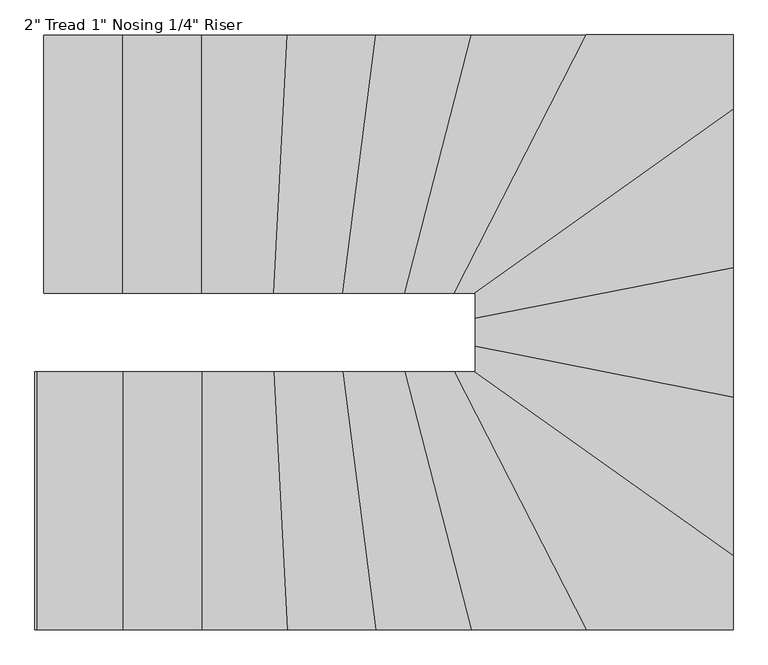
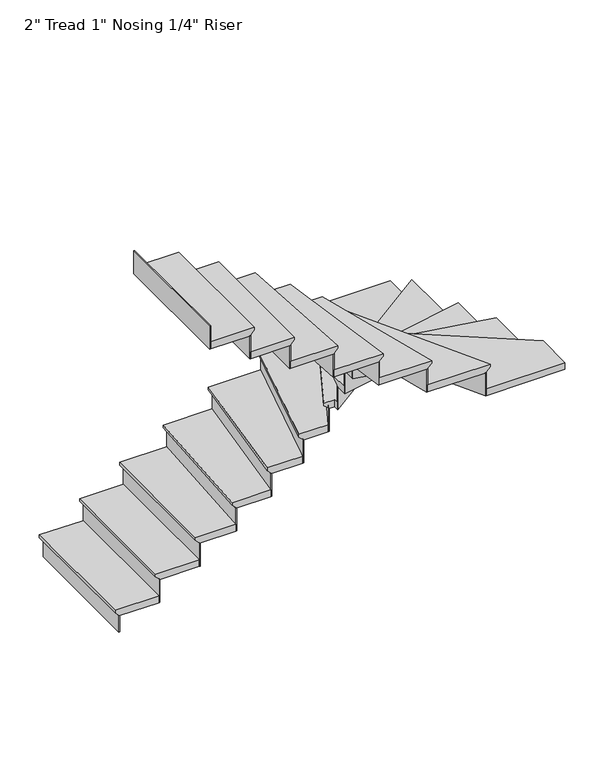
"""IFC4 building model written with IfcOpenShell, lengths in millimetres: stair flight geometry."""

from ifc_helpers import new_model, si_unit, origin, place, context, project, spatial, faceted_brep, source, transform, mapped, element, save


def stair_flight_a0830a8a(model_context):
    return source(origin(), model_context, "Body", "Brep", [
        faceted_brep([(1342.8282136, -2159.7365003, 150.2833333), (1342.8282136, -2159.7365003, 169.3333333), (1342.8282136, -1245.3365003, 169.3333333), (1342.8282136, -1245.3365003, 150.2833333), (1368.2282136, -2159.7365003, 124.8833333), (1368.2282136, -1245.3365003, 124.8833333), (1647.6282136, -2159.7365003, 169.3333333), (1647.6282136, -1245.3365003, 169.3333333), (1368.2282136, -1245.3365003, 118.5333333), (1647.6282136, -1245.3365003, 118.5333333), (1647.6282136, -2159.7365003, 118.5333333), (1368.2282136, -2159.7365003, 118.5333333)], [[[0, 1, 2, 3]], [[4, 0, 3, 5]], [[2, 1, 6, 7]], [[8, 9, 10, 11]], [[2, 7, 9, 8, 5, 3]], [[8, 11, 4, 5]], [[6, 1, 0, 4, 11, 10]], [[7, 6, 10, 9]]]),
        faceted_brep([(1368.2282136, -2159.7365003, 118.5333333), (1368.2282136, -2159.7365003, 0.0), (1374.5782136, -2159.7365003, 0.0), (1374.5782136, -2159.7365003, 118.5333333), (1368.2282136, -1245.3365003, 118.5333333), (1374.5782136, -1245.3365003, 118.5333333), (1374.5782136, -1245.3365003, 0.0), (1368.2282136, -1245.3365003, 0.0)], [[[0, 1, 2, 3]], [[4, 5, 6, 7]], [[1, 0, 4, 7]], [[2, 1, 7, 6]], [[3, 2, 6, 5]], [[0, 3, 5, 4]]]),
        faceted_brep([(1647.6282136, -2159.7365003, 287.8666667), (1647.6282136, -2159.7365003, 118.5333333), (1653.9782136, -2159.7365003, 118.5333333), (1653.9782136, -2159.7365003, 287.8666667), (1647.6282136, -1245.3365003, 287.8666667), (1653.9782136, -1245.3365003, 287.8666667), (1653.9782136, -1245.3365003, 118.5333333), (1647.6282136, -1245.3365003, 118.5333333)], [[[0, 1, 2, 3]], [[4, 5, 6, 7]], [[1, 0, 4, 7]], [[2, 1, 7, 6]], [[3, 2, 6, 5]], [[0, 3, 5, 4]]]),
        faceted_brep([(1622.2282136, -1245.3365003, 338.6666667), (1622.2282136, -2159.7365003, 338.6666667), (1927.0282136, -2159.7365003, 338.6666667), (1927.0282136, -1245.3365003, 338.6666667), (1647.6282136, -1245.3365003, 287.8666667), (1927.0282136, -1245.3365003, 287.8666667), (1927.0282136, -2159.7365003, 287.8666667), (1647.6282136, -2159.7365003, 287.8666667), (1647.6282136, -1245.3365003, 294.2166667), (1622.2282136, -1245.3365003, 319.6166667), (1647.6282136, -2159.7365003, 294.2166667), (1622.2282136, -2159.7365003, 319.6166667)], [[[0, 1, 2, 3]], [[4, 5, 6, 7]], [[0, 3, 5, 4, 8, 9]], [[4, 7, 10, 8]], [[2, 1, 11, 10, 7, 6]], [[3, 2, 6, 5]], [[11, 1, 0, 9]], [[10, 11, 9, 8]]]),
        faceted_brep([(1927.0282136, -2159.7365003, 457.2), (1927.0282136, -2159.7365003, 287.8666667), (1933.3782136, -2159.7365003, 287.8666667), (1933.3782136, -2159.7365003, 457.2), (1927.0282136, -1245.3365003, 457.2), (1933.3782136, -1245.3365003, 457.2), (1933.3782136, -1245.3365003, 287.8666667), (1927.0282136, -1245.3365003, 287.8666667)], [[[0, 1, 2, 3]], [[4, 5, 6, 7]], [[1, 0, 4, 7]], [[2, 1, 7, 6]], [[3, 2, 6, 5]], [[0, 3, 5, 4]]]),
        faceted_brep([(1901.6282136, -1245.3365003, 508.0), (1901.6282136, -2159.7365003, 508.0), (2182.6953751, -2159.7365003, 508.0), (2230.2296455, -1245.3365003, 508.0), (1927.0282136, -1245.3365003, 457.2), (2230.2296455, -1245.3365003, 457.2), (2182.6953751, -2159.7365003, 457.2), (1927.0282136, -2159.7365003, 457.2), (1927.0282136, -1245.3365003, 463.55), (1901.6282136, -1245.3365003, 488.95), (1927.0282136, -2159.7365003, 463.55), (1901.6282136, -2159.7365003, 488.95)], [[[0, 1, 2, 3]], [[4, 5, 6, 7]], [[0, 3, 5, 4, 8, 9]], [[4, 7, 10, 8]], [[2, 1, 11, 10, 7, 6]], [[3, 2, 6, 5]], [[11, 1, 0, 9]], [[10, 11, 9, 8]]]),
        faceted_brep([(2182.6953751, -2159.7365003, 626.5333333), (2182.6953751, -2159.7365003, 457.2), (2189.0539493, -2159.7365003, 457.2), (2189.0539493, -2159.7365003, 626.5333333), (2230.2296455, -1245.3365003, 626.5333333), (2236.5882197, -1245.3365003, 626.5333333), (2236.5882197, -1245.3365003, 457.2), (2230.2296455, -1245.3365003, 457.2)], [[[0, 1, 2, 3]], [[4, 5, 6, 7]], [[1, 0, 4, 7]], [[2, 1, 7, 6]], [[3, 2, 6, 5]], [[0, 3, 5, 4]]]),
        faceted_brep([(2204.7953488, -1245.3365003, 677.3333333), (2157.2610784, -2159.7365003, 677.3333333), (2426.8620749, -2159.7365003, 677.3333333), (2545.2181266, -1245.3365003, 677.3333333), (2230.2296455, -1245.3365003, 626.5333333), (2545.2181266, -1245.3365003, 626.5333333), (2426.8620749, -2159.7365003, 626.5333333), (2182.6953751, -2159.7365003, 626.5333333), (2230.2296455, -1245.3365003, 632.8833333), (2204.7953488, -1245.3365003, 658.2833333), (2182.6953751, -2159.7365003, 632.8833333), (2157.2610784, -2159.7365003, 658.2833333)], [[[0, 1, 2, 3]], [[4, 5, 6, 7]], [[0, 3, 5, 4, 8, 9]], [[4, 7, 10, 8]], [[2, 1, 11, 10, 7, 6]], [[3, 2, 6, 5]], [[11, 1, 0, 9]], [[10, 11, 9, 8]]]),
        faceted_brep([(2426.8620749, -2159.7365003, 795.8666667), (2426.8620749, -2159.7365003, 626.5333333), (2433.2650467, -2159.7365003, 626.5333333), (2433.2650467, -2159.7365003, 795.8666667), (2545.2181266, -1245.3365003, 795.8666667), (2551.6210984, -1245.3365003, 795.8666667), (2551.6210984, -1245.3365003, 626.5333333), (2545.2181266, -1245.3365003, 626.5333333)], [[[0, 1, 2, 3]], [[4, 5, 6, 7]], [[1, 0, 4, 7]], [[2, 1, 7, 6]], [[3, 2, 6, 5]], [[0, 3, 5, 4]]]),
        faceted_brep([(2519.6062395, -1245.3365003, 846.6666667), (2401.2501878, -2159.7365003, 846.6666667), (2648.4892974, -2159.7365003, 846.6666667), (2883.6197448, -1245.3365003, 846.6666667), (2545.2181266, -1245.3365003, 795.8666667), (2883.6197448, -1245.3365003, 795.8666667), (2648.4892974, -2159.7365003, 795.8666667), (2426.8620749, -2159.7365003, 795.8666667), (2545.2181266, -1245.3365003, 802.2166667), (2519.6062395, -1245.3365003, 827.6166667), (2426.8620749, -2159.7365003, 802.2166667), (2401.2501878, -2159.7365003, 827.6166667)], [[[0, 1, 2, 3]], [[4, 5, 6, 7]], [[0, 3, 5, 4, 8, 9]], [[4, 7, 10, 8]], [[2, 1, 11, 10, 7, 6]], [[3, 2, 6, 5]], [[11, 1, 0, 9]], [[10, 11, 9, 8]]]),
        faceted_brep([(2648.4892974, -2159.7365003, 965.2), (2648.4892974, -2159.7365003, 795.8666667), (2655.0458743, -2159.7365003, 795.8666667), (2655.0458743, -2159.7365003, 965.2), (2883.6197448, -1245.3365003, 965.2), (2890.1763217, -1245.3365003, 965.2), (2890.1763217, -1245.3365003, 795.8666667), (2883.6197448, -1245.3365003, 795.8666667)], [[[0, 1, 2, 3]], [[4, 5, 6, 7]], [[1, 0, 4, 7]], [[2, 1, 7, 6]], [[3, 2, 6, 5]], [[0, 3, 5, 4]]]),
        faceted_brep([(2857.3934373, -1245.3365003, 1016.0), (2622.2629899, -2159.7365003, 1016.0), (2824.8359335, -2159.7365003, 1016.0), (3293.6605548, -1245.3365003, 1016.0), (2883.6197448, -1245.3365003, 965.2), (3293.6605548, -1245.3365003, 965.2), (2824.8359335, -2159.7365003, 965.2), (2648.4892974, -2159.7365003, 965.2), (2883.6197448, -1245.3365003, 971.55), (2857.3934373, -1245.3365003, 996.95), (2648.4892974, -2159.7365003, 971.55), (2622.2629899, -2159.7365003, 996.95)], [[[0, 1, 2, 3]], [[4, 5, 6, 7]], [[0, 3, 5, 4, 8, 9]], [[4, 7, 10, 8]], [[2, 1, 11, 10, 7, 6]], [[3, 2, 6, 5]], [[11, 1, 0, 9]], [[10, 11, 9, 8]]]),
        faceted_brep([(2824.8359335, -2159.7365003, 1134.5333333), (2824.8359335, -2159.7365003, 965.2), (2831.9719166, -2159.7365003, 965.2), (2831.9719166, -2159.7365003, 1134.5333333), (3293.6605548, -1245.3365003, 1134.5333333), (3300.7965379, -1245.3365003, 1134.5333333), (3300.7965379, -1245.3365003, 965.2), (3293.6605548, -1245.3365003, 965.2)], [[[0, 1, 2, 3]], [[4, 5, 6, 7]], [[1, 0, 4, 7]], [[2, 1, 7, 6]], [[3, 2, 6, 5]], [[0, 3, 5, 4]]]),
        faceted_brep([(3784.9599055, -1539.017634, 1185.3333333), (3784.9599055, -1245.3365003, 1185.3333333), (3265.1166223, -1245.3365003, 1185.3333333), (2796.2920009, -2159.7365003, 1185.3333333), (2870.5599055, -2159.7365003, 1185.3333333), (2870.5599055, -2189.2915832, 1185.3333333), (3784.9599055, -1245.3365003, 1134.5333333), (3784.9599055, -1539.017634, 1134.5333333), (2870.5599055, -2189.2915832, 1134.5333333), (2870.5599055, -2159.7365003, 1134.5333333), (2824.8359335, -2159.7365003, 1134.5333333), (3293.6605548, -1245.3365003, 1134.5333333), (3293.6605548, -1245.3365003, 1140.8833333), (3265.1166223, -1245.3365003, 1166.2833333), (2824.8359335, -2159.7365003, 1140.8833333), (2796.2920009, -2159.7365003, 1166.2833333)], [[[0, 1, 2, 3, 4, 5]], [[6, 7, 8, 9, 10, 11]], [[1, 0, 7, 6]], [[2, 1, 6, 11, 12, 13]], [[11, 10, 14, 12]], [[4, 3, 15, 14, 10, 9]], [[5, 4, 9, 8]], [[0, 5, 8, 7]], [[15, 3, 2, 13]], [[14, 15, 13, 12]]]),
        faceted_brep([(2870.5599055, -2189.2915832, 1303.8666667), (2870.5599055, -2189.2915832, 1134.5333333), (2870.5599055, -2197.083558, 1134.5333333), (2870.5599055, -2197.083558, 1303.8666667), (3784.9599055, -1539.017634, 1303.8666667), (3784.9599055, -1546.8096088, 1303.8666667), (3784.9599055, -1546.8096088, 1134.5333333), (3784.9599055, -1539.017634, 1134.5333333)], [[[0, 1, 2, 3]], [[4, 5, 6, 7]], [[1, 0, 4, 7]], [[2, 1, 7, 6]], [[3, 2, 6, 5]], [[0, 3, 5, 4]]]),
        faceted_brep([(3784.9599055, -1507.8497349, 1354.6666667), (2870.5599055, -2158.123684, 1354.6666667), (2870.5599055, -2275.7456703, 1354.6666667), (3784.9599055, -2095.5048139, 1354.6666667), (3784.9599055, -1539.017634, 1303.8666667), (3784.9599055, -2095.5048139, 1303.8666667), (2870.5599055, -2275.7456703, 1303.8666667), (2870.5599055, -2189.2915832, 1303.8666667), (3784.9599055, -1539.017634, 1310.2166667), (3784.9599055, -1507.8497349, 1335.6166667), (2870.5599055, -2189.2915832, 1310.2166667), (2870.5599055, -2158.123684, 1335.6166667)], [[[0, 1, 2, 3]], [[4, 5, 6, 7]], [[0, 3, 5, 4, 8, 9]], [[4, 7, 10, 8]], [[2, 1, 11, 10, 7, 6]], [[3, 2, 6, 5]], [[11, 1, 0, 9]], [[10, 11, 9, 8]]]),
        faceted_brep([(2870.5599055, -2275.7456703, 1473.2), (2870.5599055, -2275.7456703, 1303.8666667), (2870.5599055, -2282.2178557, 1303.8666667), (2870.5599055, -2282.2178557, 1473.2), (3784.9599055, -2095.5048139, 1473.2), (3784.9599055, -2101.9769994, 1473.2), (3784.9599055, -2101.9769994, 1303.8666667), (3784.9599055, -2095.5048139, 1303.8666667)], [[[0, 1, 2, 3]], [[4, 5, 6, 7]], [[1, 0, 4, 7]], [[2, 1, 7, 6]], [[3, 2, 6, 5]], [[0, 3, 5, 4]]]),
        faceted_brep([(3784.9599055, -2069.6160722, 1524.0), (2870.5599055, -2249.8569285, 1524.0), (2870.5599055, -2374.9048139, 1524.0), (3784.9599055, -2555.1456703, 1524.0), (3784.9599055, -2095.5048139, 1473.2), (3784.9599055, -2555.1456703, 1473.2), (2870.5599055, -2374.9048139, 1473.2), (2870.5599055, -2275.7456703, 1473.2), (3784.9599055, -2095.5048139, 1479.55), (3784.9599055, -2069.6160722, 1504.95), (2870.5599055, -2275.7456703, 1479.55), (2870.5599055, -2249.8569285, 1504.95)], [[[0, 1, 2, 3]], [[4, 5, 6, 7]], [[0, 3, 5, 4, 8, 9]], [[4, 7, 10, 8]], [[2, 1, 11, 10, 7, 6]], [[3, 2, 6, 5]], [[11, 1, 0, 9]], [[10, 11, 9, 8]]]),
        faceted_brep([(2870.5599055, -2374.9048139, 1642.5333333), (2870.5599055, -2374.9048139, 1473.2), (2870.5599055, -2381.3769994, 1473.2), (2870.5599055, -2381.3769994, 1642.5333333), (3784.9599055, -2555.1456703, 1642.5333333), (3784.9599055, -2561.6178557, 1642.5333333), (3784.9599055, -2561.6178557, 1473.2), (3784.9599055, -2555.1456703, 1473.2)], [[[0, 1, 2, 3]], [[4, 5, 6, 7]], [[1, 0, 4, 7]], [[2, 1, 7, 6]], [[3, 2, 6, 5]], [[0, 3, 5, 4]]]),
        faceted_brep([(3784.9599055, -2529.2569285, 1693.3333333), (2870.5599055, -2349.0160722, 1693.3333333), (2870.5599055, -2439.1365003, 1693.3333333), (2824.464431, -2439.1365003, 1693.3333333), (3784.9599055, -3122.191165, 1693.3333333), (3784.9599055, -2555.1456703, 1642.5333333), (3784.9599055, -3122.191165, 1642.5333333), (2824.464431, -2439.1365003, 1642.5333333), (2870.5599055, -2439.1365003, 1642.5333333), (2870.5599055, -2374.9048139, 1642.5333333), (3784.9599055, -2555.1456703, 1648.8833333), (3784.9599055, -2529.2569285, 1674.2833333), (2870.5599055, -2374.9048139, 1648.8833333), (2870.5599055, -2349.0160722, 1674.2833333)], [[[0, 1, 2, 3, 4]], [[5, 6, 7, 8, 9]], [[0, 4, 6, 5, 10, 11]], [[5, 9, 12, 10]], [[2, 1, 13, 12, 9, 8]], [[3, 2, 8, 7]], [[4, 3, 7, 6]], [[13, 1, 0, 11]], [[12, 13, 11, 10]]]),
        faceted_brep([(2824.464431, -2439.1365003, 1811.8666667), (2824.464431, -2439.1365003, 1642.5333333), (2813.5075385, -2439.1365003, 1642.5333333), (2813.5075385, -2439.1365003, 1811.8666667), (3784.9599055, -3122.191165, 1811.8666667), (3784.9599055, -3129.9831398, 1811.8666667), (3784.9599055, -3129.9831398, 1642.5333333), (3784.9599055, -3122.191165, 1642.5333333)], [[[0, 1, 2, 3]], [[4, 5, 6, 7]], [[1, 0, 4, 7]], [[2, 1, 7, 6]], [[3, 2, 6, 5]], [[0, 3, 5, 4]]]),
        faceted_brep([(3236.5726897, -3353.5365003, 1862.6666667), (3784.9599055, -3353.5365003, 1862.6666667), (3784.9599055, -3091.0232658, 1862.6666667), (2868.2920009, -2439.1365003, 1862.6666667), (2767.7480684, -2439.1365003, 1862.6666667), (3784.9599055, -3353.5365003, 1811.8666667), (3236.5726897, -3353.5365003, 1811.8666667), (2767.7480684, -2439.1365003, 1811.8666667), (2824.464431, -2439.1365003, 1811.8666667), (3784.9599055, -3122.191165, 1811.8666667), (3784.9599055, -3122.191165, 1818.2166667), (3784.9599055, -3091.0232658, 1843.6166667), (2824.464431, -2439.1365003, 1818.2166667), (2868.2920009, -2439.1365003, 1843.6166667)], [[[0, 1, 2, 3, 4]], [[5, 6, 7, 8, 9]], [[1, 0, 6, 5]], [[2, 1, 5, 9, 10, 11]], [[9, 8, 12, 10]], [[4, 3, 13, 12, 8, 7]], [[0, 4, 7, 6]], [[13, 3, 2, 11]], [[12, 13, 11, 10]]]),
        faceted_brep([(2767.7480684, -2439.1365003, 1981.2), (2767.7480684, -2439.1365003, 1811.8666667), (2760.6120853, -2439.1365003, 1811.8666667), (2760.6120853, -2439.1365003, 1981.2), (3236.5726897, -3353.5365003, 1981.2), (3229.4367066, -3353.5365003, 1981.2), (3229.4367066, -3353.5365003, 1811.8666667), (3236.5726897, -3353.5365003, 1811.8666667)], [[[0, 1, 2, 3]], [[4, 5, 6, 7]], [[1, 0, 4, 7]], [[2, 1, 7, 6]], [[3, 2, 6, 5]], [[0, 3, 5, 4]]]),
        faceted_brep([(3265.1166223, -3353.5365003, 2032.0), (2796.2920009, -2439.1365003, 2032.0), (2596.0366825, -2439.1365003, 2032.0), (2831.1671299, -3353.5365003, 2032.0), (3236.5726897, -3353.5365003, 1981.2), (2831.1671299, -3353.5365003, 1981.2), (2596.0366825, -2439.1365003, 1981.2), (2767.7480684, -2439.1365003, 1981.2), (3236.5726897, -3353.5365003, 1987.55), (3265.1166223, -3353.5365003, 2012.95), (2767.7480684, -2439.1365003, 1987.55), (2796.2920009, -2439.1365003, 2012.95)], [[[0, 1, 2, 3]], [[4, 5, 6, 7]], [[0, 3, 5, 4, 8, 9]], [[4, 7, 10, 8]], [[2, 1, 11, 10, 7, 6]], [[3, 2, 6, 5]], [[11, 1, 0, 9]], [[10, 11, 9, 8]]]),
        faceted_brep([(2596.0366825, -2439.1365003, 2150.5333333), (2596.0366825, -2439.1365003, 1981.2), (2589.4801056, -2439.1365003, 1981.2), (2589.4801056, -2439.1365003, 2150.5333333), (2831.1671299, -3353.5365003, 2150.5333333), (2824.610553, -3353.5365003, 2150.5333333), (2824.610553, -3353.5365003, 1981.2), (2831.1671299, -3353.5365003, 1981.2)], [[[0, 1, 2, 3]], [[4, 5, 6, 7]], [[1, 0, 4, 7]], [[2, 1, 7, 6]], [[3, 2, 6, 5]], [[0, 3, 5, 4]]]),
        faceted_brep([(2857.3934373, -3353.5365003, 2201.3333333), (2622.2629899, -2439.1365003, 2201.3333333), (2375.6383007, -2439.1365003, 2201.3333333), (2493.9943524, -3353.5365003, 2201.3333333), (2831.1671299, -3353.5365003, 2150.5333333), (2493.9943524, -3353.5365003, 2150.5333333), (2375.6383007, -2439.1365003, 2150.5333333), (2596.0366825, -2439.1365003, 2150.5333333), (2831.1671299, -3353.5365003, 2156.8833333), (2857.3934373, -3353.5365003, 2182.2833333), (2596.0366825, -2439.1365003, 2156.8833333), (2622.2629899, -2439.1365003, 2182.2833333)], [[[0, 1, 2, 3]], [[4, 5, 6, 7]], [[0, 3, 5, 4, 8, 9]], [[4, 7, 10, 8]], [[2, 1, 11, 10, 7, 6]], [[3, 2, 6, 5]], [[11, 1, 0, 9]], [[10, 11, 9, 8]]]),
        faceted_brep([(2375.6383007, -2439.1365003, 2319.8666667), (2375.6383007, -2439.1365003, 2150.5333333), (2369.2353289, -2439.1365003, 2150.5333333), (2369.2353289, -2439.1365003, 2319.8666667), (2493.9943524, -3353.5365003, 2319.8666667), (2487.5913806, -3353.5365003, 2319.8666667), (2487.5913806, -3353.5365003, 2150.5333333), (2493.9943524, -3353.5365003, 2150.5333333)], [[[0, 1, 2, 3]], [[4, 5, 6, 7]], [[1, 0, 4, 7]], [[2, 1, 7, 6]], [[3, 2, 6, 5]], [[0, 3, 5, 4]]]),
        faceted_brep([(2519.6062395, -3353.5365003, 2370.6666667), (2401.2501878, -2439.1365003, 2370.6666667), (2131.8267818, -2439.1365003, 2370.6666667), (2179.3610522, -3353.5365003, 2370.6666667), (2493.9943524, -3353.5365003, 2319.8666667), (2179.3610522, -3353.5365003, 2319.8666667), (2131.8267818, -2439.1365003, 2319.8666667), (2375.6383007, -2439.1365003, 2319.8666667), (2493.9943524, -3353.5365003, 2326.2166667), (2519.6062395, -3353.5365003, 2351.6166667), (2375.6383007, -2439.1365003, 2326.2166667), (2401.2501878, -2439.1365003, 2351.6166667)], [[[0, 1, 2, 3]], [[4, 5, 6, 7]], [[0, 3, 5, 4, 8, 9]], [[4, 7, 10, 8]], [[2, 1, 11, 10, 7, 6]], [[3, 2, 6, 5]], [[11, 1, 0, 9]], [[10, 11, 9, 8]]]),
        faceted_brep([(2131.8267818, -2439.1365003, 2489.2), (2131.8267818, -2439.1365003, 2319.8666667), (2125.4682076, -2439.1365003, 2319.8666667), (2125.4682076, -2439.1365003, 2489.2), (2179.3610522, -3353.5365003, 2489.2), (2173.002478, -3353.5365003, 2489.2), (2173.002478, -3353.5365003, 2319.8666667), (2179.3610522, -3353.5365003, 2319.8666667)], [[[0, 1, 2, 3]], [[4, 5, 6, 7]], [[1, 0, 4, 7]], [[2, 1, 7, 6]], [[3, 2, 6, 5]], [[0, 3, 5, 4]]]),
        faceted_brep([(2204.7953488, -3353.5365003, 2540.0), (2157.2610784, -2439.1365003, 2540.0), (1876.2282136, -2439.1365003, 2540.0), (1876.2282136, -3353.5365003, 2540.0), (2179.3610522, -3353.5365003, 2489.2), (1876.2282136, -3353.5365003, 2489.2), (1876.2282136, -2439.1365003, 2489.2), (2131.8267818, -2439.1365003, 2489.2), (2179.3610522, -3353.5365003, 2495.55), (2204.7953488, -3353.5365003, 2520.95), (2131.8267818, -2439.1365003, 2495.55), (2157.2610784, -2439.1365003, 2520.95)], [[[0, 1, 2, 3]], [[4, 5, 6, 7]], [[0, 3, 5, 4, 8, 9]], [[4, 7, 10, 8]], [[2, 1, 11, 10, 7, 6]], [[3, 2, 6, 5]], [[11, 1, 0, 9]], [[10, 11, 9, 8]]]),
        faceted_brep([(1876.2282136, -2439.1365003, 2658.5333333), (1876.2282136, -2439.1365003, 2489.2), (1869.8782136, -2439.1365003, 2489.2), (1869.8782136, -2439.1365003, 2658.5333333), (1876.2282136, -3353.5365003, 2658.5333333), (1869.8782136, -3353.5365003, 2658.5333333), (1869.8782136, -3353.5365003, 2489.2), (1876.2282136, -3353.5365003, 2489.2)], [[[0, 1, 2, 3]], [[4, 5, 6, 7]], [[1, 0, 4, 7]], [[2, 1, 7, 6]], [[3, 2, 6, 5]], [[0, 3, 5, 4]]]),
        faceted_brep([(1901.6282136, -3353.5365003, 2709.3333333), (1901.6282136, -2439.1365003, 2709.3333333), (1596.8282136, -2439.1365003, 2709.3333333), (1596.8282136, -3353.5365003, 2709.3333333), (1876.2282136, -3353.5365003, 2658.5333333), (1596.8282136, -3353.5365003, 2658.5333333), (1596.8282136, -2439.1365003, 2658.5333333), (1876.2282136, -2439.1365003, 2658.5333333), (1876.2282136, -3353.5365003, 2664.8833333), (1901.6282136, -3353.5365003, 2690.2833333), (1876.2282136, -2439.1365003, 2664.8833333), (1901.6282136, -2439.1365003, 2690.2833333)], [[[0, 1, 2, 3]], [[4, 5, 6, 7]], [[0, 3, 5, 4, 8, 9]], [[4, 7, 10, 8]], [[2, 1, 11, 10, 7, 6]], [[3, 2, 6, 5]], [[11, 1, 0, 9]], [[10, 11, 9, 8]]]),
        faceted_brep([(1596.8282136, -2439.1365003, 2827.8666667), (1596.8282136, -2439.1365003, 2658.5333333), (1590.4782136, -2439.1365003, 2658.5333333), (1590.4782136, -2439.1365003, 2827.8666667), (1596.8282136, -3353.5365003, 2827.8666667), (1590.4782136, -3353.5365003, 2827.8666667), (1590.4782136, -3353.5365003, 2658.5333333), (1596.8282136, -3353.5365003, 2658.5333333)], [[[0, 1, 2, 3]], [[4, 5, 6, 7]], [[1, 0, 4, 7]], [[2, 1, 7, 6]], [[3, 2, 6, 5]], [[0, 3, 5, 4]]]),
        faceted_brep([(1317.4282136, -2439.1365003, 2997.2), (1317.4282136, -2439.1365003, 2827.8666667), (1311.0782136, -2439.1365003, 2827.8666667), (1311.0782136, -2439.1365003, 2997.2), (1317.4282136, -3353.5365003, 2997.2), (1311.0782136, -3353.5365003, 2997.2), (1311.0782136, -3353.5365003, 2827.8666667), (1317.4282136, -3353.5365003, 2827.8666667)], [[[0, 1, 2, 3]], [[4, 5, 6, 7]], [[1, 0, 4, 7]], [[2, 1, 7, 6]], [[3, 2, 6, 5]], [[0, 3, 5, 4]]]),
        faceted_brep([(1622.2282136, -3353.5365003, 2878.6666667), (1622.2282136, -2439.1365003, 2878.6666667), (1317.4282136, -2439.1365003, 2878.6666667), (1317.4282136, -3353.5365003, 2878.6666667), (1596.8282136, -3353.5365003, 2827.8666667), (1317.4282136, -3353.5365003, 2827.8666667), (1317.4282136, -2439.1365003, 2827.8666667), (1596.8282136, -2439.1365003, 2827.8666667), (1596.8282136, -3353.5365003, 2834.2166667), (1622.2282136, -3353.5365003, 2859.6166667), (1596.8282136, -2439.1365003, 2834.2166667), (1622.2282136, -2439.1365003, 2859.6166667)], [[[0, 1, 2, 3]], [[4, 5, 6, 7]], [[0, 3, 5, 4, 8, 9]], [[4, 7, 10, 8]], [[2, 1, 11, 10, 7, 6]], [[3, 2, 6, 5]], [[11, 1, 0, 9]], [[10, 11, 9, 8]]]),
    ])


if __name__ == "__main__":
    model = new_model("IFC4")
    model_context = context("Model", 3, world=origin())
    ifc_project = project(units=[si_unit("LENGTHUNIT", "METRE", prefix="MILLI")], contexts=[model_context])
    site = spatial("IfcSite", under=ifc_project)
    building = spatial("IfcBuilding", under=site)
    placement = place(None, origin())
    stair_flight_shape = stair_flight_a0830a8a(model_context)
    element("IfcStairFlight", 1, ObjectType="2\" Tread 1\" Nosing 1/4\" Riser", at=placement, inside=building, context=model_context, shape_type="MappedRepresentation", body=[
        mapped(stair_flight_shape, transform((0.0, 0.0, 0.0), x_axis=(1.0, 0.0, 0.0), y_axis=(0.0, 1.0, 0.0), z_axis=(0.0, 0.0, 1.0))),
    ])
    save(model, "model.ifc")
